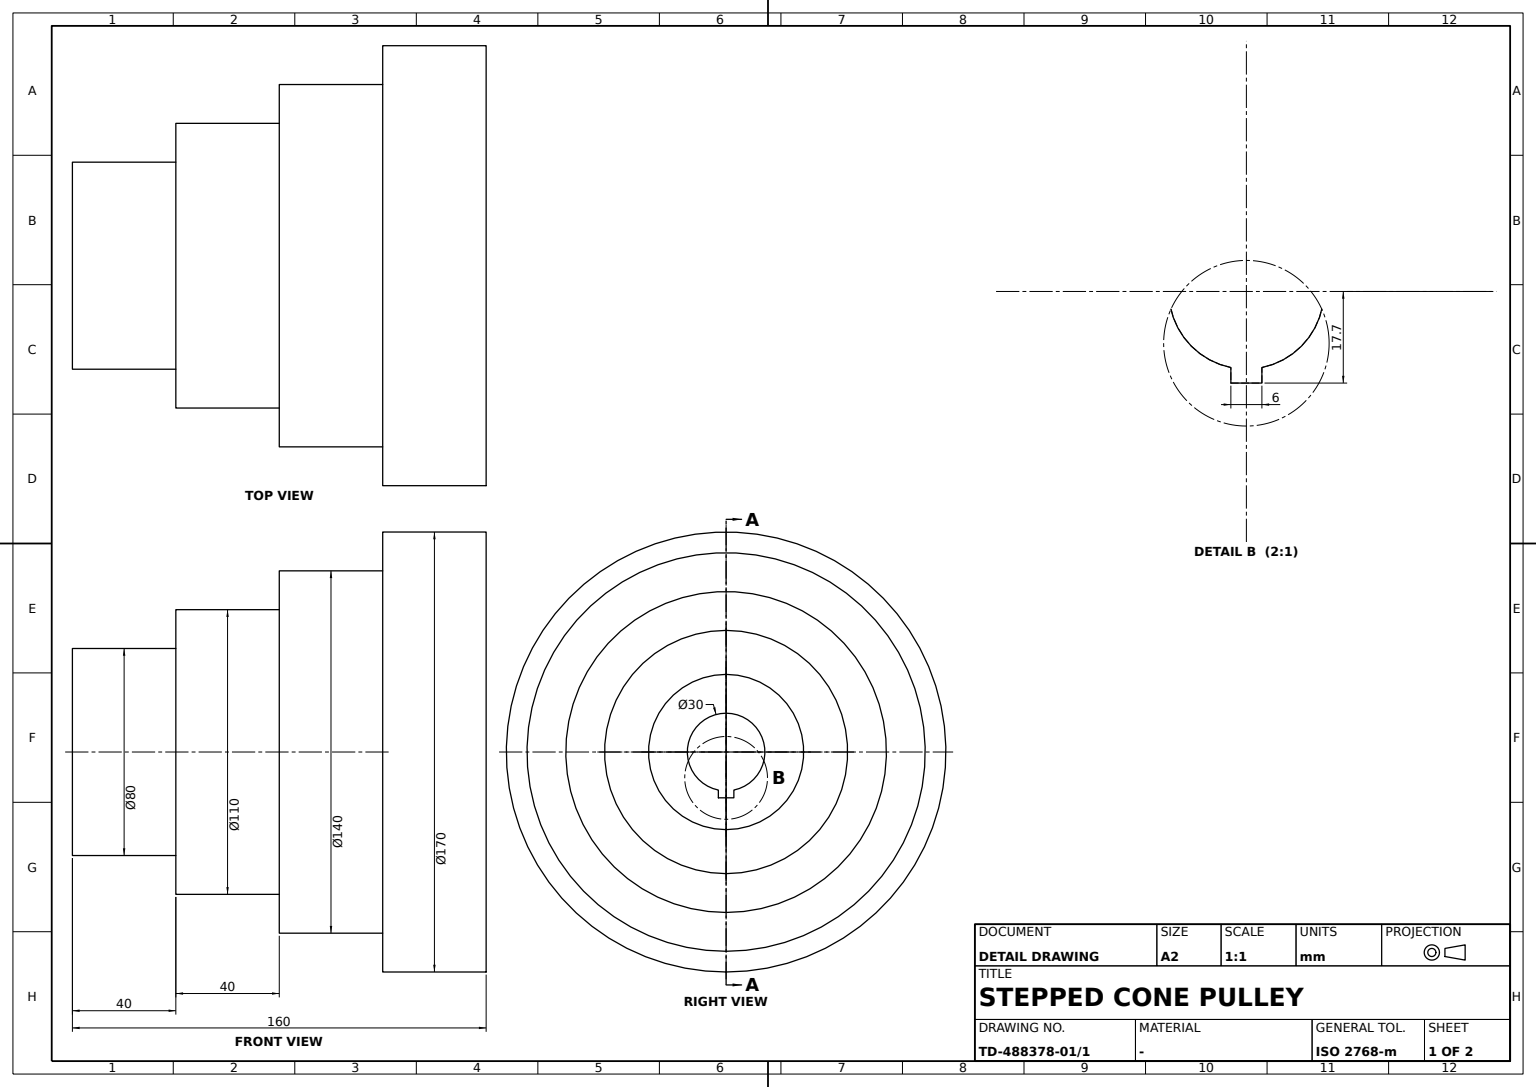
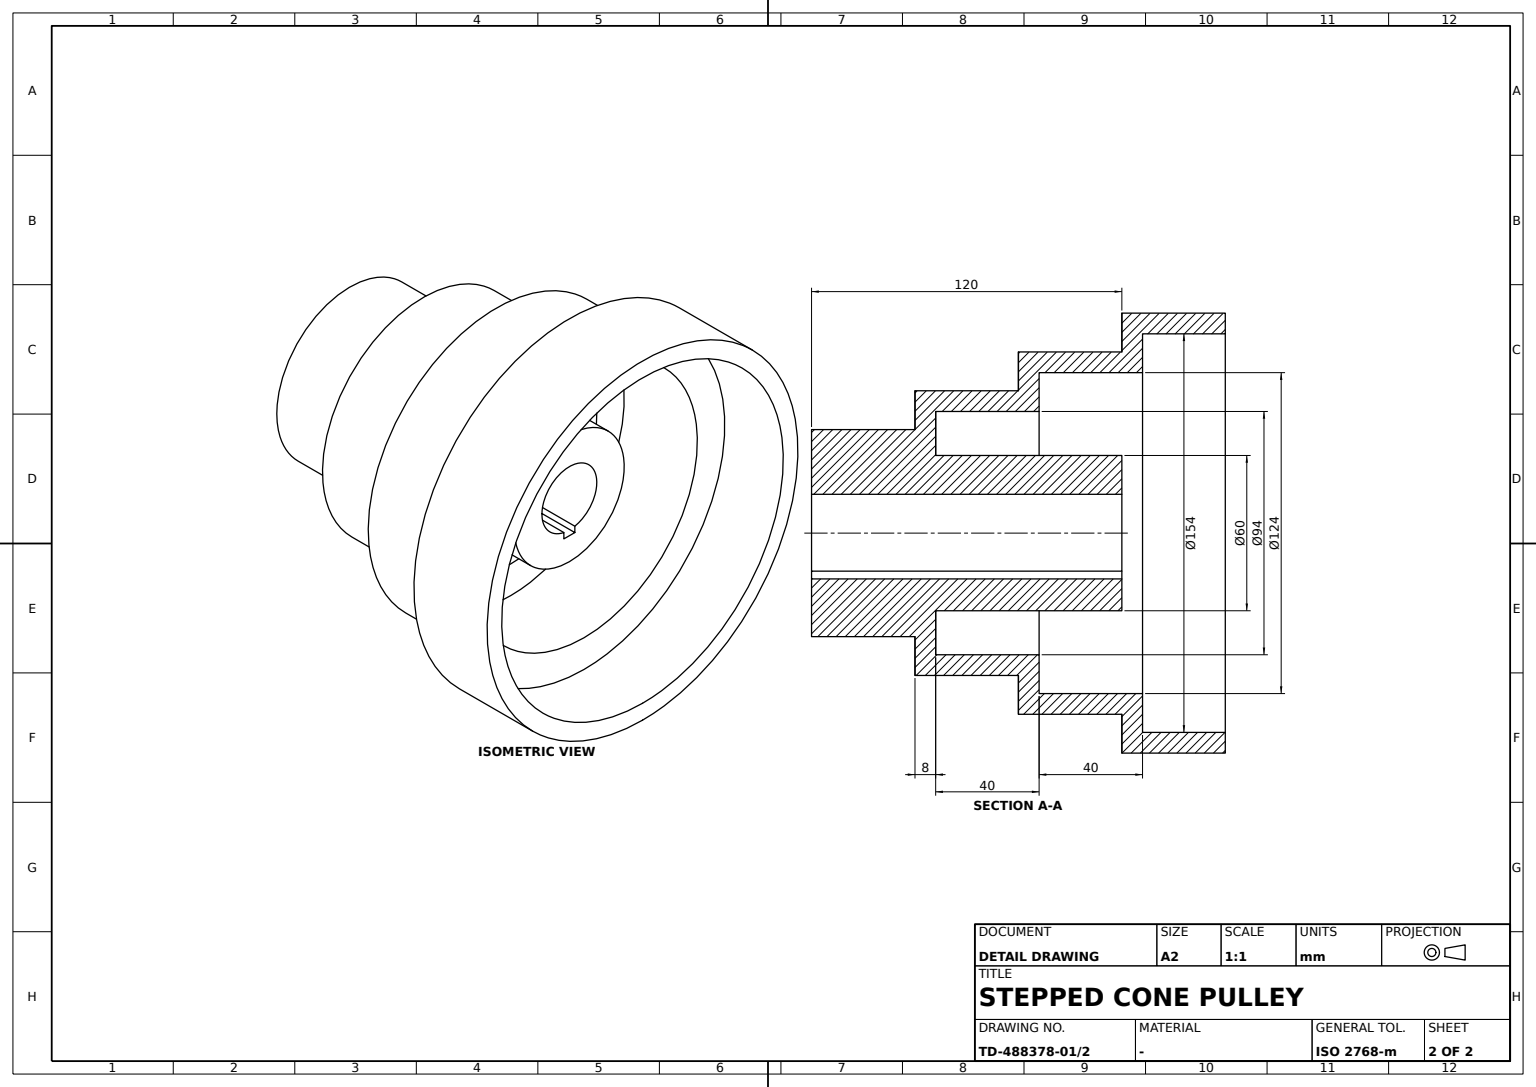
CATIA V5 part; units mm, degrees
sketch "Sketch1" plane through (0, 0, 0) normal (1, 0, 0) x (0, 1, 0)
  point P0 (0, 15)
  line L0 (0, 15) -> (120, 15)
  line L1 (120, 70) -> (80, 70)
  line L2 (80, 70) -> (80, 55)
  line L3 (80, 55) -> (40, 55)
  line L4 (40, 55) -> (40, 40)
  line L5 (40, 40) -> (0, 40)
  point P1 (0, 40)
  line L6 (0, 40) -> (0, 15)
  line L7 (154.591, 0) -> (-165.4713, 0) construction
  point P2 (154.591, 0)
  line L8 (120, 70) -> (120, 85)
  line L9 (120, 85) -> (160, 85)
  line L10 (120, 15) -> (120, 30)
  line L11 (120, 30) -> (48, 30)
  line L12 (48, 30) -> (48, 47)
  line L13 (48, 47) -> (88, 47)
  line L14 (88, 47) -> (88, 62)
  line L15 (88, 62) -> (128, 62)
  line L16 (128, 62) -> (128, 77)
  line L17 (128, 77) -> (160, 77)
  line L18 (160, 77) -> (160, 85)
  dimension "distance L5 L7" = 40
  dimension "distance L0 L7" = 15
  dimension "length L0" = 120
  dimension "length L5" = 40
  dimension "length L3" = 40
  dimension "length L1" = 40
  dimension "distance L3 L7" = 55
  dimension "distance L1 L7" = 70
  dimension "distance L9 L7" = 85
  dimension "distance L11 L7" = 30
  dimension "distance L9 L17" = 8
  dimension "length L9" = 40
  dimension "distance L15 L1" = 8
  dimension "distance L13 L3" = 8
  dimension "distance L16 L8" = 8
  dimension "distance L14 L2" = 8
  dimension "distance L12 L4" = 8
  constraint coincidence P0 y-axis
  constraint coincidence P1 y-axis
  constraint coincidence P2 x-axis
  constraint horizontal L0 x-axis
  constraint horizontal L1 x-axis
  constraint horizontal L3 x-axis
  constraint horizontal L5 x-axis
  constraint horizontal L7 x-axis
  constraint horizontal L9 x-axis
  constraint horizontal L11 x-axis
  constraint horizontal L13 x-axis
  constraint horizontal L15 x-axis
  constraint horizontal L17 x-axis
  constraint vertical L2 y-axis
  constraint vertical L4 y-axis
  constraint vertical L6 y-axis
  constraint vertical L8 y-axis
  constraint vertical L10 y-axis
  constraint vertical L12 y-axis
  constraint vertical L14 y-axis
  constraint vertical L16 y-axis
  constraint vertical L18 y-axis
revolve "Shaft1" add sketch "Sketch1" angle 360 about L7
sketch "Sketch2" plane through (0, 0, 0) normal (0, -1, 0) x (1, 0, 0)
  circle A0 centre (0, 0) radius 15 construction
  arc A1 (-3, -14.6969) -> (3, -14.6969) centre (0, 0) ccw
  point P0 (0, -15)
  line L0 (3, -14.6969) -> (3, -17.6969)
  line L1 (3, -17.6969) -> (-3, -17.6969)
  line L2 (-3, -17.6969) -> (-3, -14.6969)
  point P1 (3, -14.6969)
  point P2 (-3, -14.6969)
  dimension "length L1" = 6
  dimension "length L0" = 3
  constraint coincidence P0 A0
  constraint coincidence P0 y-axis
  constraint coincidence A0 P1
  constraint coincidence A0 P2
  constraint vertical L0 y-axis
  constraint vertical L2 y-axis
  constraint horizontal L1 x-axis
  constraint equidistance L0 L2 P0
  constraint symmetry L2 L0 y-axis
extrude "Pocket1" cut sketch "Sketch2" against normal through all
